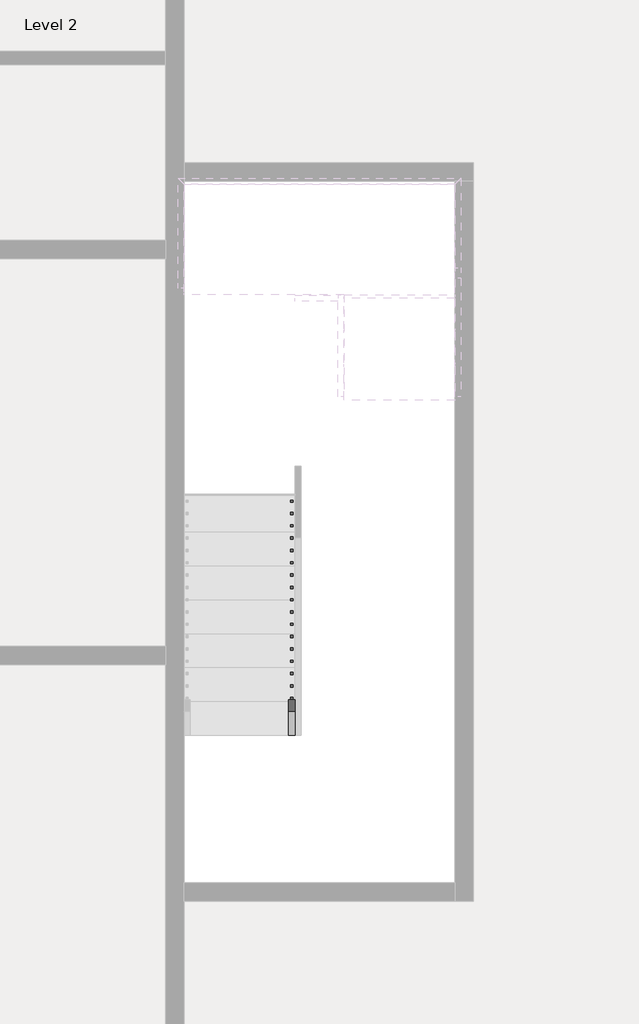
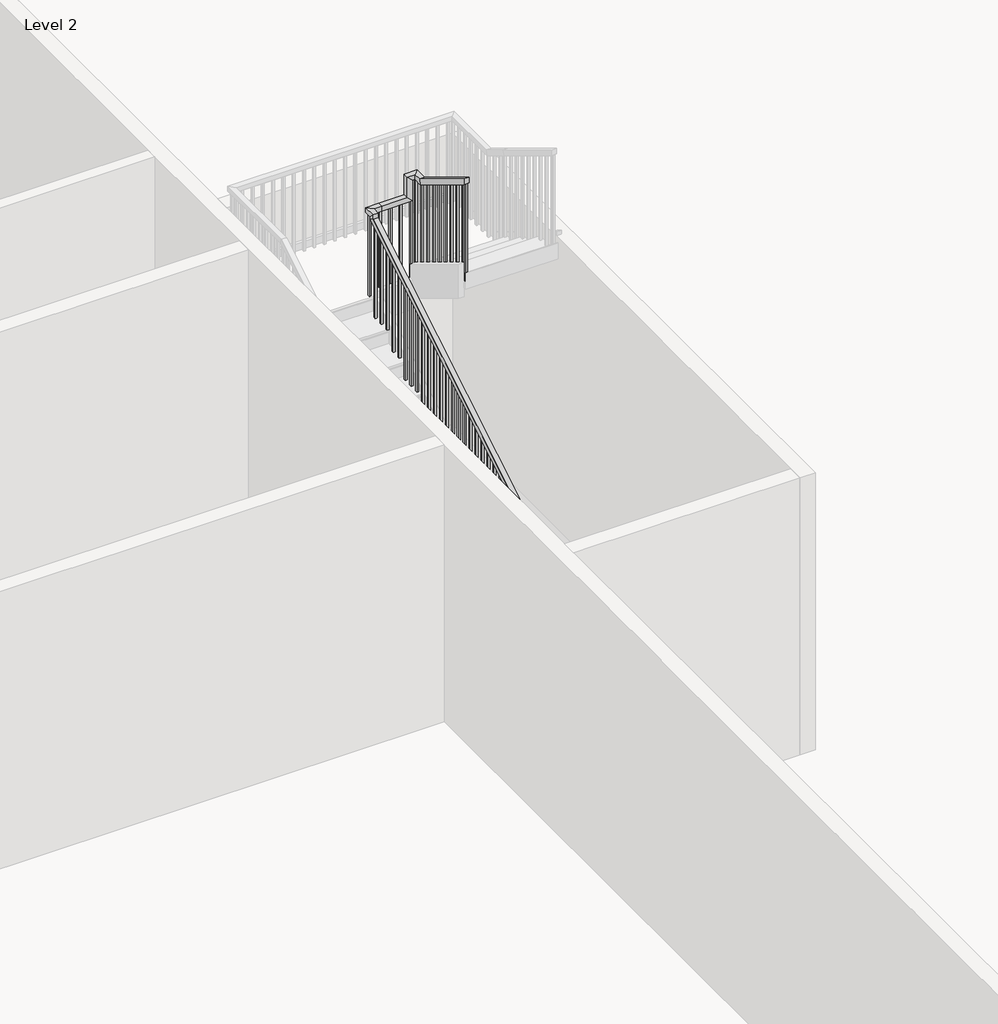
# One storey, part 5 of 8: 1 railing.
"""IFC4 building model written with IfcOpenShell, lengths in millimetres."""

from ifc_helpers import new_model, si_unit, frame, origin, place, context, project, spatial, polyline, outline, extrude, faceted_brep, element, save

model = new_model("IFC4")

# Units and contexts
model_context = context("Model", 3, world=origin())
ifc_project = project(units=[si_unit("LENGTHUNIT", "METRE", prefix="MILLI")], contexts=[model_context])

# Site, building, storey
site = spatial("IfcSite", under=ifc_project)
building = spatial("IfcBuilding", under=site)
storey = spatial("IfcBuildingStorey", under=building, Name="Level 2", Elevation=28282.6172466)

# Railing
placement = place(None, origin())
element("IfcRailing", 1, ObjectType="Handrail - Rectangular", at=placement, inside=storey, context=model_context, shape_type="SolidModel", body=[
    faceted_brep([(-2753.8415084, -23154.3851539, 29366.3505799), (-2753.8415084, -23154.3851539, 29306.9491197), (-2703.0415084, -23154.3851539, 29306.9491197), (-2703.0415084, -23154.3851539, 29366.3505799), (-2753.8415084, -19598.3851539, 31521.5020951), (-2753.8415084, -19547.5851539, 31492.8885136), (-2703.0415084, -19547.5851539, 31492.8885136), (-2703.0415084, -19598.3851539, 31521.5020951), (-2753.8415084, -19598.3851539, 31567.6839133), (-2753.8415084, -19547.5851539, 31516.8839133), (-2703.0415084, -19547.5851539, 31516.8839133), (-2703.0415084, -19598.3851539, 31567.6839133), (-2753.8415084, -19471.3851539, 31567.6839133), (-2753.8415084, -19471.3851539, 31516.8839133), (-2703.0415084, -19522.1851539, 31516.8839133), (-2703.0415084, -19522.1851539, 31567.6839133), (-2626.8415084, -19471.3851539, 31567.6839133), (-2626.8415084, -19471.3851539, 31516.8839133), (-2626.8415084, -19522.1851539, 31516.8839133), (-2626.8415084, -19522.1851539, 31567.6839133), (-2372.8415084, -19471.3851539, 31567.6839133), (-2322.0415084, -19471.3851539, 31516.8839133), (-2322.0415084, -19522.1851539, 31516.8839133), (-2372.8415084, -19522.1851539, 31567.6839133), (-2372.8415084, -19471.3851539, 31783.1990648), (-2322.0415084, -19471.3851539, 31732.3990648), (-2322.0415084, -19522.1851539, 31732.3990648), (-2372.8415084, -19522.1851539, 31783.1990648), (-2245.8415084, -19471.3851539, 31783.1990648), (-2245.8415084, -19471.3851539, 31732.3990648), (-2296.6415084, -19522.1851539, 31732.3990648), (-2296.6415084, -19522.1851539, 31783.1990648), (-2245.8415084, -19598.3851539, 31783.1990648), (-2245.8415084, -19612.5775633, 31732.3990648), (-2296.6415084, -19612.5775633, 31732.3990648), (-2296.6415084, -19598.3851539, 31783.1990648), (-2245.8415084, -20360.3851539, 32245.0172466), (-2296.6415084, -20360.3851539, 32245.0172466), (-2296.6415084, -20360.3851539, 32185.6157863), (-2245.8415084, -20360.3851539, 32185.6157863)], [[[0, 1, 2, 3]], [[1, 0, 4, 5]], [[2, 1, 5, 6]], [[3, 2, 6, 7]], [[0, 3, 7, 4]], [[5, 4, 8, 9]], [[6, 5, 9, 10]], [[7, 6, 10, 11]], [[4, 7, 11, 8]], [[9, 8, 12, 13]], [[10, 9, 13, 14]], [[11, 10, 14, 15]], [[8, 11, 15, 12]], [[13, 12, 16, 17]], [[14, 13, 17, 18]], [[15, 14, 18, 19]], [[12, 15, 19, 16]], [[17, 16, 20, 21]], [[18, 17, 21, 22]], [[19, 18, 22, 23]], [[16, 19, 23, 20]], [[21, 20, 24, 25]], [[22, 21, 25, 26]], [[23, 22, 26, 27]], [[20, 23, 27, 24]], [[25, 24, 28, 29]], [[26, 25, 29, 30]], [[27, 26, 30, 31]], [[24, 27, 31, 28]], [[29, 28, 32, 33]], [[30, 29, 33, 34]], [[31, 30, 34, 35]], [[28, 31, 35, 32]], [[36, 37, 38, 39]], [[33, 32, 36, 39]], [[34, 33, 39, 38]], [[35, 34, 38, 37]], [[32, 35, 37, 36]]]),
    extrude(outline(polyline([(-20319.1101539, 32160.6006348), (-20300.0601539, 32149.0551803), (-20300.0601539, 31161.2839133), (-20319.1101539, 31161.2839133), (-20319.1101539, 32160.6006348)])), frame((-2280.7665084, 0.0, 0.0), z_axis=(1.0, 0.0, 0.0), x_axis=(0.0, 1.0, 0.0)), (0.0, 0.0, 1.0), 19.05),
    extrude(outline(polyline([(-20217.5101539, 32099.0248773), (-20198.4601539, 32087.4794227), (-20198.4601539, 31161.2839133), (-20217.5101539, 31161.2839133), (-20217.5101539, 32099.0248773)])), frame((-2280.7665084, 0.0, 0.0), z_axis=(1.0, 0.0, 0.0), x_axis=(0.0, 1.0, 0.0)), (0.0, 0.0, 1.0), 19.05),
    extrude(outline(polyline([(-20115.9101539, 32037.4491197), (-20096.8601539, 32025.9036651), (-20096.8601539, 31161.2839133), (-20115.9101539, 31161.2839133), (-20115.9101539, 32037.4491197)])), frame((-2280.7665084, 0.0, 0.0), z_axis=(1.0, 0.0, 0.0), x_axis=(0.0, 1.0, 0.0)), (0.0, 0.0, 1.0), 19.05),
    extrude(outline(polyline([(-20014.3101539, 31975.8733621), (-19995.2601539, 31964.3279076), (-19995.2601539, 30991.9505799), (-20014.3101539, 30991.9505799), (-20014.3101539, 31975.8733621)])), frame((-2280.7665084, 0.0, 0.0), z_axis=(1.0, 0.0, 0.0), x_axis=(0.0, 1.0, 0.0)), (0.0, 0.0, 1.0), 19.05),
    extrude(outline(polyline([(-19912.7101539, 31914.2976045), (-19893.6601539, 31902.75215), (-19893.6601539, 30991.9505799), (-19912.7101539, 30991.9505799), (-19912.7101539, 31914.2976045)])), frame((-2280.7665084, 0.0, 0.0), z_axis=(1.0, 0.0, 0.0), x_axis=(0.0, 1.0, 0.0)), (0.0, 0.0, 1.0), 19.05),
    extrude(outline(polyline([(-19811.1101539, 31852.721847), (-19792.0601539, 31841.1763924), (-19792.0601539, 30991.9505799), (-19811.1101539, 30991.9505799), (-19811.1101539, 31852.721847)])), frame((-2280.7665084, 0.0, 0.0), z_axis=(1.0, 0.0, 0.0), x_axis=(0.0, 1.0, 0.0)), (0.0, 0.0, 1.0), 19.05),
    extrude(outline(polyline([(-19709.5101539, 31791.1460894), (-19690.4601539, 31779.6006348), (-19690.4601539, 30822.6172466), (-19709.5101539, 30822.6172466), (-19709.5101539, 31791.1460894)])), frame((-2280.7665084, 0.0, 0.0), z_axis=(1.0, 0.0, 0.0), x_axis=(0.0, 1.0, 0.0)), (0.0, 0.0, 1.0), 19.05),
    extrude(outline(polyline([(-19607.9101539, 31729.5703318), (-19588.8601539, 31718.0248773), (-19588.8601539, 30822.6172466), (-19607.9101539, 30822.6172466), (-19607.9101539, 31729.5703318)])), frame((-2280.7665084, 0.0, 0.0), z_axis=(1.0, 0.0, 0.0), x_axis=(0.0, 1.0, 0.0)), (0.0, 0.0, 1.0), 19.05),
    extrude(outline(polyline([(-2331.5665084, -19506.3101539), (-2331.5665084, -19487.2601539), (-2312.5165084, -19487.2601539), (-2312.5165084, -19506.3101539), (-2331.5665084, -19506.3101539)])), frame((0.0, 0.0, 30653.2839133), z_axis=(0.0, 0.0, 1.0), x_axis=(1.0, 0.0, 0.0)), (0.0, 0.0, 1.0), 1079.1151515),
    extrude(outline(polyline([(-2433.1665084, -19506.3101539), (-2433.1665084, -19487.2601539), (-2414.1165084, -19487.2601539), (-2414.1165084, -19506.3101539), (-2433.1665084, -19506.3101539)])), frame((0.0, 0.0, 30653.2839133), z_axis=(0.0, 0.0, 1.0), x_axis=(1.0, 0.0, 0.0)), (0.0, 0.0, 1.0), 863.6),
    extrude(outline(polyline([(-2534.7665084, -19506.3101539), (-2534.7665084, -19487.2601539), (-2515.7165084, -19487.2601539), (-2515.7165084, -19506.3101539), (-2534.7665084, -19506.3101539)])), frame((0.0, 0.0, 30653.2839133), z_axis=(0.0, 0.0, 1.0), x_axis=(1.0, 0.0, 0.0)), (0.0, 0.0, 1.0), 863.6),
    extrude(outline(polyline([(-2636.3665084, -19506.3101539), (-2636.3665084, -19487.2601539), (-2617.3165084, -19487.2601539), (-2617.3165084, -19506.3101539), (-2636.3665084, -19506.3101539)])), frame((0.0, 0.0, 30653.2839133), z_axis=(0.0, 0.0, 1.0), x_axis=(1.0, 0.0, 0.0)), (0.0, 0.0, 1.0), 863.6),
    extrude(outline(polyline([(-19607.9101539, 31456.3279076), (-19588.8601539, 31467.8733621), (-19588.8601539, 30483.9505799), (-19607.9101539, 30483.9505799), (-19607.9101539, 31456.3279076)])), frame((-2737.9665084, 0.0, 0.0), z_axis=(1.0, 0.0, 0.0), x_axis=(0.0, 1.0, 0.0)), (0.0, 0.0, 1.0), 19.05),
    extrude(outline(polyline([(-19709.5101539, 31394.75215), (-19690.4601539, 31406.2976045), (-19690.4601539, 30483.9505799), (-19709.5101539, 30483.9505799), (-19709.5101539, 31394.75215)])), frame((-2737.9665084, 0.0, 0.0), z_axis=(1.0, 0.0, 0.0), x_axis=(0.0, 1.0, 0.0)), (0.0, 0.0, 1.0), 19.05),
    extrude(outline(polyline([(-19811.1101539, 31333.1763924), (-19792.0601539, 31344.721847), (-19792.0601539, 30483.9505799), (-19811.1101539, 30483.9505799), (-19811.1101539, 31333.1763924)])), frame((-2737.9665084, 0.0, 0.0), z_axis=(1.0, 0.0, 0.0), x_axis=(0.0, 1.0, 0.0)), (0.0, 0.0, 1.0), 19.05),
    extrude(outline(polyline([(-19912.7101539, 31271.6006348), (-19893.6601539, 31283.1460894), (-19893.6601539, 30314.6172466), (-19912.7101539, 30314.6172466), (-19912.7101539, 31271.6006348)])), frame((-2737.9665084, 0.0, 0.0), z_axis=(1.0, 0.0, 0.0), x_axis=(0.0, 1.0, 0.0)), (0.0, 0.0, 1.0), 19.05),
    extrude(outline(polyline([(-20014.3101539, 31210.0248773), (-19995.2601539, 31221.5703318), (-19995.2601539, 30314.6172466), (-20014.3101539, 30314.6172466), (-20014.3101539, 31210.0248773)])), frame((-2737.9665084, 0.0, 0.0), z_axis=(1.0, 0.0, 0.0), x_axis=(0.0, 1.0, 0.0)), (0.0, 0.0, 1.0), 19.05),
    extrude(outline(polyline([(-20115.9101539, 31148.4491197), (-20096.8601539, 31159.9945742), (-20096.8601539, 30145.2839133), (-20115.9101539, 30145.2839133), (-20115.9101539, 31148.4491197)])), frame((-2737.9665084, 0.0, 0.0), z_axis=(1.0, 0.0, 0.0), x_axis=(0.0, 1.0, 0.0)), (0.0, 0.0, 1.0), 19.05),
    extrude(outline(polyline([(-20217.5101539, 31086.8733621), (-20198.4601539, 31098.4188167), (-20198.4601539, 30145.2839133), (-20217.5101539, 30145.2839133), (-20217.5101539, 31086.8733621)])), frame((-2737.9665084, 0.0, 0.0), z_axis=(1.0, 0.0, 0.0), x_axis=(0.0, 1.0, 0.0)), (0.0, 0.0, 1.0), 19.05),
    extrude(outline(polyline([(-20319.1101539, 31025.2976045), (-20300.0601539, 31036.8430591), (-20300.0601539, 30145.2839133), (-20319.1101539, 30145.2839133), (-20319.1101539, 31025.2976045)])), frame((-2737.9665084, 0.0, 0.0), z_axis=(1.0, 0.0, 0.0), x_axis=(0.0, 1.0, 0.0)), (0.0, 0.0, 1.0), 19.05),
    extrude(outline(polyline([(-20420.7101539, 30963.721847), (-20401.6601539, 30975.2673015), (-20401.6601539, 29975.9505799), (-20420.7101539, 29975.9505799), (-20420.7101539, 30963.721847)])), frame((-2737.9665084, 0.0, 0.0), z_axis=(1.0, 0.0, 0.0), x_axis=(0.0, 1.0, 0.0)), (0.0, 0.0, 1.0), 19.05),
    extrude(outline(polyline([(-20522.3101539, 30902.1460894), (-20503.2601539, 30913.6915439), (-20503.2601539, 29975.9505799), (-20522.3101539, 29975.9505799), (-20522.3101539, 30902.1460894)])), frame((-2737.9665084, 0.0, 0.0), z_axis=(1.0, 0.0, 0.0), x_axis=(0.0, 1.0, 0.0)), (0.0, 0.0, 1.0), 19.05),
    extrude(outline(polyline([(-20623.9101539, 30840.5703318), (-20604.8601539, 30852.1157863), (-20604.8601539, 29975.9505799), (-20623.9101539, 29975.9505799), (-20623.9101539, 30840.5703318)])), frame((-2737.9665084, 0.0, 0.0), z_axis=(1.0, 0.0, 0.0), x_axis=(0.0, 1.0, 0.0)), (0.0, 0.0, 1.0), 19.05),
    extrude(outline(polyline([(-20725.5101539, 30778.9945742), (-20706.4601539, 30790.5400288), (-20706.4601539, 29806.6172466), (-20725.5101539, 29806.6172466), (-20725.5101539, 30778.9945742)])), frame((-2737.9665084, 0.0, 0.0), z_axis=(1.0, 0.0, 0.0), x_axis=(0.0, 1.0, 0.0)), (0.0, 0.0, 1.0), 19.05),
    extrude(outline(polyline([(-20827.1101539, 30717.4188167), (-20808.0601539, 30728.9642712), (-20808.0601539, 29806.6172466), (-20827.1101539, 29806.6172466), (-20827.1101539, 30717.4188167)])), frame((-2737.9665084, 0.0, 0.0), z_axis=(1.0, 0.0, 0.0), x_axis=(0.0, 1.0, 0.0)), (0.0, 0.0, 1.0), 19.05),
    extrude(outline(polyline([(-20928.7101539, 30655.8430591), (-20909.6601539, 30667.3885136), (-20909.6601539, 29806.6172466), (-20928.7101539, 29806.6172466), (-20928.7101539, 30655.8430591)])), frame((-2737.9665084, 0.0, 0.0), z_axis=(1.0, 0.0, 0.0), x_axis=(0.0, 1.0, 0.0)), (0.0, 0.0, 1.0), 19.05),
    extrude(outline(polyline([(-21030.3101539, 30594.2673015), (-21011.2601539, 30605.812756), (-21011.2601539, 29637.2839133), (-21030.3101539, 29637.2839133), (-21030.3101539, 30594.2673015)])), frame((-2737.9665084, 0.0, 0.0), z_axis=(1.0, 0.0, 0.0), x_axis=(0.0, 1.0, 0.0)), (0.0, 0.0, 1.0), 19.05),
    extrude(outline(polyline([(-21131.9101539, 30532.6915439), (-21112.8601539, 30544.2369985), (-21112.8601539, 29637.2839133), (-21131.9101539, 29637.2839133), (-21131.9101539, 30532.6915439)])), frame((-2737.9665084, 0.0, 0.0), z_axis=(1.0, 0.0, 0.0), x_axis=(0.0, 1.0, 0.0)), (0.0, 0.0, 1.0), 19.05),
    extrude(outline(polyline([(-21233.5101539, 30471.1157863), (-21214.4601539, 30482.6612409), (-21214.4601539, 29467.9505799), (-21233.5101539, 29467.9505799), (-21233.5101539, 30471.1157863)])), frame((-2737.9665084, 0.0, 0.0), z_axis=(1.0, 0.0, 0.0), x_axis=(0.0, 1.0, 0.0)), (0.0, 0.0, 1.0), 19.05),
    extrude(outline(polyline([(-21335.1101539, 30409.5400288), (-21316.0601539, 30421.0854833), (-21316.0601539, 29467.9505799), (-21335.1101539, 29467.9505799), (-21335.1101539, 30409.5400288)])), frame((-2737.9665084, 0.0, 0.0), z_axis=(1.0, 0.0, 0.0), x_axis=(0.0, 1.0, 0.0)), (0.0, 0.0, 1.0), 19.05),
    extrude(outline(polyline([(-21436.7101539, 30347.9642712), (-21417.6601539, 30359.5097257), (-21417.6601539, 29467.9505799), (-21436.7101539, 29467.9505799), (-21436.7101539, 30347.9642712)])), frame((-2737.9665084, 0.0, 0.0), z_axis=(1.0, 0.0, 0.0), x_axis=(0.0, 1.0, 0.0)), (0.0, 0.0, 1.0), 19.05),
    extrude(outline(polyline([(-21538.3101539, 30286.3885136), (-21519.2601539, 30297.9339682), (-21519.2601539, 29298.6172466), (-21538.3101539, 29298.6172466), (-21538.3101539, 30286.3885136)])), frame((-2737.9665084, 0.0, 0.0), z_axis=(1.0, 0.0, 0.0), x_axis=(0.0, 1.0, 0.0)), (0.0, 0.0, 1.0), 19.05),
    extrude(outline(polyline([(-21639.9101539, 30224.812756), (-21620.8601539, 30236.3582106), (-21620.8601539, 29298.6172466), (-21639.9101539, 29298.6172466), (-21639.9101539, 30224.812756)])), frame((-2737.9665084, 0.0, 0.0), z_axis=(1.0, 0.0, 0.0), x_axis=(0.0, 1.0, 0.0)), (0.0, 0.0, 1.0), 19.05),
    extrude(outline(polyline([(-21741.5101539, 30163.2369985), (-21722.4601539, 30174.782453), (-21722.4601539, 29298.6172466), (-21741.5101539, 29298.6172466), (-21741.5101539, 30163.2369985)])), frame((-2737.9665084, 0.0, 0.0), z_axis=(1.0, 0.0, 0.0), x_axis=(0.0, 1.0, 0.0)), (0.0, 0.0, 1.0), 19.05),
    extrude(outline(polyline([(-21843.1101539, 30101.6612409), (-21824.0601539, 30113.2066954), (-21824.0601539, 29129.2839133), (-21843.1101539, 29129.2839133), (-21843.1101539, 30101.6612409)])), frame((-2737.9665084, 0.0, 0.0), z_axis=(1.0, 0.0, 0.0), x_axis=(0.0, 1.0, 0.0)), (0.0, 0.0, 1.0), 19.05),
    extrude(outline(polyline([(-21944.7101539, 30040.0854833), (-21925.6601539, 30051.6309379), (-21925.6601539, 29129.2839133), (-21944.7101539, 29129.2839133), (-21944.7101539, 30040.0854833)])), frame((-2737.9665084, 0.0, 0.0), z_axis=(1.0, 0.0, 0.0), x_axis=(0.0, 1.0, 0.0)), (0.0, 0.0, 1.0), 19.05),
    extrude(outline(polyline([(-22046.3101539, 29978.5097257), (-22027.2601539, 29990.0551803), (-22027.2601539, 29129.2839133), (-22046.3101539, 29129.2839133), (-22046.3101539, 29978.5097257)])), frame((-2737.9665084, 0.0, 0.0), z_axis=(1.0, 0.0, 0.0), x_axis=(0.0, 1.0, 0.0)), (0.0, 0.0, 1.0), 19.05),
    extrude(outline(polyline([(-22147.9101539, 29916.9339682), (-22128.8601539, 29928.4794227), (-22128.8601539, 28959.9505799), (-22147.9101539, 28959.9505799), (-22147.9101539, 29916.9339682)])), frame((-2737.9665084, 0.0, 0.0), z_axis=(1.0, 0.0, 0.0), x_axis=(0.0, 1.0, 0.0)), (0.0, 0.0, 1.0), 19.05),
    extrude(outline(polyline([(-22249.5101539, 29855.3582106), (-22230.4601539, 29866.9036651), (-22230.4601539, 28959.9505799), (-22249.5101539, 28959.9505799), (-22249.5101539, 29855.3582106)])), frame((-2737.9665084, 0.0, 0.0), z_axis=(1.0, 0.0, 0.0), x_axis=(0.0, 1.0, 0.0)), (0.0, 0.0, 1.0), 19.05),
    extrude(outline(polyline([(-22351.1101539, 29793.782453), (-22332.0601539, 29805.3279076), (-22332.0601539, 28790.6172466), (-22351.1101539, 28790.6172466), (-22351.1101539, 29793.782453)])), frame((-2737.9665084, 0.0, 0.0), z_axis=(1.0, 0.0, 0.0), x_axis=(0.0, 1.0, 0.0)), (0.0, 0.0, 1.0), 19.05),
    extrude(outline(polyline([(-22452.7101539, 29732.2066954), (-22433.6601539, 29743.75215), (-22433.6601539, 28790.6172466), (-22452.7101539, 28790.6172466), (-22452.7101539, 29732.2066954)])), frame((-2737.9665084, 0.0, 0.0), z_axis=(1.0, 0.0, 0.0), x_axis=(0.0, 1.0, 0.0)), (0.0, 0.0, 1.0), 19.05),
    extrude(outline(polyline([(-22554.3101539, 29670.6309379), (-22535.2601539, 29682.1763924), (-22535.2601539, 28790.6172466), (-22554.3101539, 28790.6172466), (-22554.3101539, 29670.6309379)])), frame((-2737.9665084, 0.0, 0.0), z_axis=(1.0, 0.0, 0.0), x_axis=(0.0, 1.0, 0.0)), (0.0, 0.0, 1.0), 19.05),
    extrude(outline(polyline([(-22655.9101539, 29609.0551803), (-22636.8601539, 29620.6006348), (-22636.8601539, 28621.2839133), (-22655.9101539, 28621.2839133), (-22655.9101539, 29609.0551803)])), frame((-2737.9665084, 0.0, 0.0), z_axis=(1.0, 0.0, 0.0), x_axis=(0.0, 1.0, 0.0)), (0.0, 0.0, 1.0), 19.05),
    extrude(outline(polyline([(-22757.5101539, 29547.4794227), (-22738.4601539, 29559.0248773), (-22738.4601539, 28621.2839133), (-22757.5101539, 28621.2839133), (-22757.5101539, 29547.4794227)])), frame((-2737.9665084, 0.0, 0.0), z_axis=(1.0, 0.0, 0.0), x_axis=(0.0, 1.0, 0.0)), (0.0, 0.0, 1.0), 19.05),
    extrude(outline(polyline([(-22859.1101539, 29485.9036651), (-22840.0601539, 29497.4491197), (-22840.0601539, 28621.2839133), (-22859.1101539, 28621.2839133), (-22859.1101539, 29485.9036651)])), frame((-2737.9665084, 0.0, 0.0), z_axis=(1.0, 0.0, 0.0), x_axis=(0.0, 1.0, 0.0)), (0.0, 0.0, 1.0), 19.05),
    extrude(outline(polyline([(-22960.7101539, 29424.3279076), (-22941.6601539, 29435.8733621), (-22941.6601539, 28451.9505799), (-22960.7101539, 28451.9505799), (-22960.7101539, 29424.3279076)])), frame((-2737.9665084, 0.0, 0.0), z_axis=(1.0, 0.0, 0.0), x_axis=(0.0, 1.0, 0.0)), (0.0, 0.0, 1.0), 19.05),
    extrude(outline(polyline([(-23062.3101539, 29362.75215), (-23043.2601539, 29374.2976045), (-23043.2601539, 28451.9505799), (-23062.3101539, 28451.9505799), (-23062.3101539, 29362.75215)])), frame((-2737.9665084, 0.0, 0.0), z_axis=(1.0, 0.0, 0.0), x_axis=(0.0, 1.0, 0.0)), (0.0, 0.0, 1.0), 19.05),
    extrude(outline(polyline([(-2280.7665084, -19506.3101539), (-2280.7665084, -19487.2601539), (-2261.7165084, -19487.2601539), (-2261.7165084, -19506.3101539), (-2280.7665084, -19506.3101539)])), frame((0.0, 0.0, 30653.2839133), z_axis=(0.0, 0.0, 1.0), x_axis=(1.0, 0.0, 0.0)), (0.0, 0.0, 1.0), 1079.1151515),
    extrude(outline(polyline([(-2718.9165084, -19506.3101539), (-2737.9665084, -19506.3101539), (-2737.9665084, -19487.2601539), (-2718.9165084, -19487.2601539), (-2718.9165084, -19506.3101539)])), frame((0.0, 0.0, 30653.2839133), z_axis=(0.0, 0.0, 1.0), x_axis=(1.0, 0.0, 0.0)), (0.0, 0.0, 1.0), 863.6),
    extrude(outline(polyline([(-20360.3851539, 32185.6157863), (-20341.3351539, 32174.0703318), (-20341.3351539, 31161.2839133), (-20360.3851539, 31161.2839133), (-20360.3851539, 32185.6157863)])), frame((-2280.7665084, 0.0, 0.0), z_axis=(1.0, 0.0, 0.0), x_axis=(0.0, 1.0, 0.0)), (0.0, 0.0, 1.0), 19.05),
    extrude(outline(polyline([(-23154.3851539, 29306.9491197), (-23135.3351539, 29318.4945742), (-23135.3351539, 28451.9505799), (-23154.3851539, 28451.9505799), (-23154.3851539, 29306.9491197)])), frame((-2737.9665084, 0.0, 0.0), z_axis=(1.0, 0.0, 0.0), x_axis=(0.0, 1.0, 0.0)), (0.0, 0.0, 1.0), 19.05),
])

save(model, "model.ifc")

# Revit data of these elements
# Type "Handrail - Rectangular"
#   Assembly Code = "C2010400"
#   built-in parameter 1008612 = 0.0416667 (stored number, unit not read)
#   built-in parameter 1008611 = 0.0416667 (stored number, unit not read)
#   built-in parameter 1008609 = 0.333333 (stored number, unit not read)
#   built-in parameter 1008604 = 0.166667 (stored number, unit not read)
#   built-in parameter 1008603 = 0.166667 (stored number, unit not read)
#   Railing Height = 3' - 0"
#   built-in parameter 1008630 = 2
#   built-in parameter 1008610 = 2
#   built-in parameter 1008618 = Baluster - Square : 3/4"
# Element 1 (IfcRailing, "Handrail - Rectangular")
#   Phase Created = New Construction
